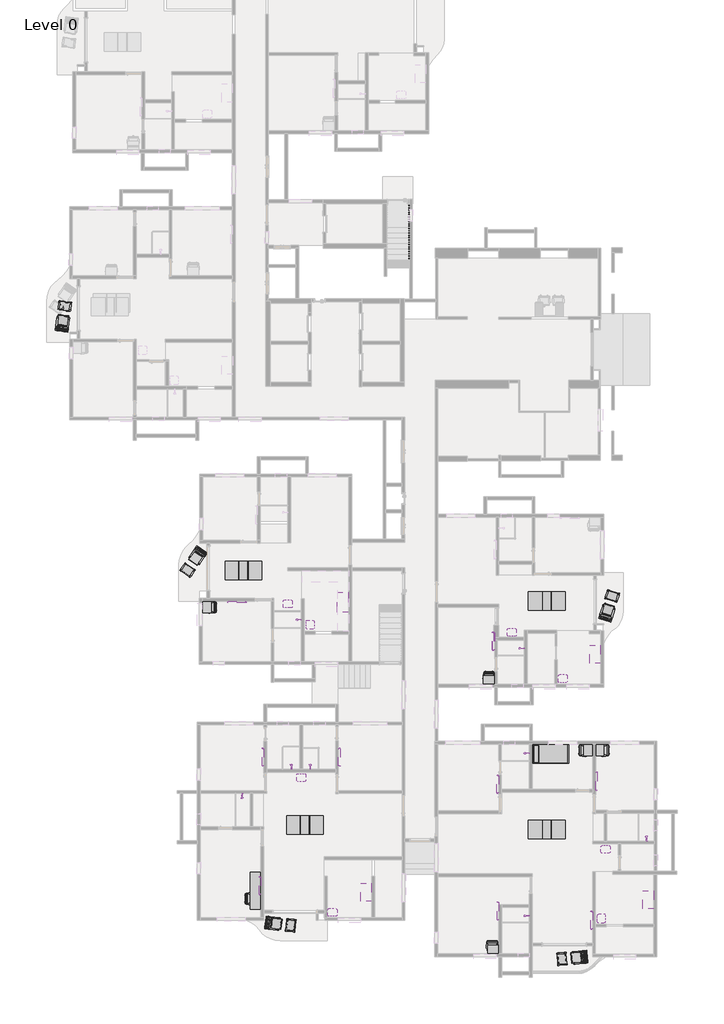
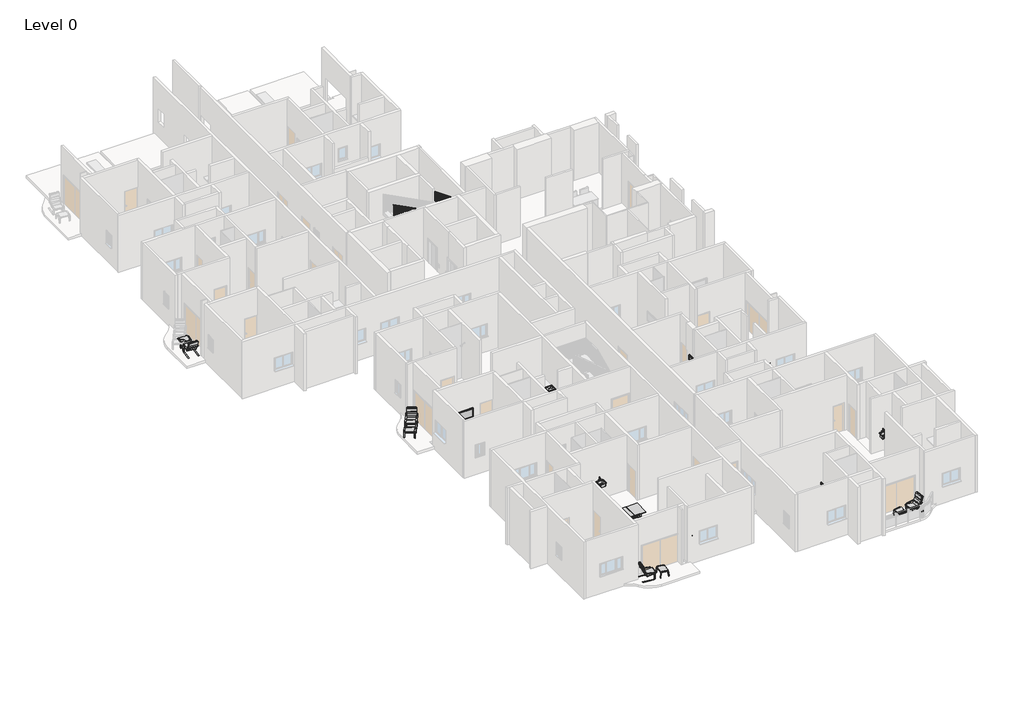
# One storey, part 13 of 14: 32 furniture elements, 16 flow terminals, 4 proxies, 1 railing.
"""IFC4 building model written with IfcOpenShell, lengths in millimetres."""

from ifc_helpers import new_model, si_unit, frame, origin, place, context, project, spatial, polyline, outline, extrude, faceted_brep, transform, mapped, element, save
from components import cook_top_2_0915_x_500mm_892363c5, cook_top_2_1000_x_525mm_c9be7e00, flow_terminal_f629513f, plumbing_fixtures_shower_head_metal_shower_head_9404fff0, furniture_b0964881, furniture_8acf2248, escritorio_de_estudiante_de_600x740mm_600_x_460_x_740mm_3f482482, furniture_bed_2_1040x1981x330mm_twin_f17094d1, furniture_chair_desk_w_armrest_2_635x686x380mm_bb362225, furniture_0b97a49d, furniture_table_dining_w_chairs_rectangular_2000x1000x750mm_b8cbee69

model = new_model("IFC4")

# Units and contexts
model_context = context("Model", 3, world=origin())
ifc_project = project(units=[si_unit("LENGTHUNIT", "METRE", prefix="MILLI")], contexts=[model_context])

# Site, building, storey
site = spatial("IfcSite", under=ifc_project)
building = spatial("IfcBuilding", under=site)
storey = spatial("IfcBuildingStorey", under=building, Name="Level 0", Elevation=0.0)

# Proxies
placement = place(None, origin())
cook_top_2_0915_x_500mm_shape = cook_top_2_0915_x_500mm_892363c5(model_context)
element("IfcBuildingElementProxy", 1, Name="Cook_Top_(2) : 0915 x 500mm", ObjectType="Cook_Top_(2) : 0915 x 500mm", at=placement, inside=storey, context=model_context, shape_type="MappedRepresentation", body=[
    mapped(cook_top_2_0915_x_500mm_shape, transform((-23700.2563508, 13394.0304681, 457.2), x_axis=(0.0, 1.0, 0.0), y_axis=(-1.0, 0.0, 0.0), z_axis=(0.0, 0.0, 1.0))),
])
element("IfcBuildingElementProxy", 2, Name="Cook_Top_(2) : 0915 x 500mm", ObjectType="Cook_Top_(2) : 0915 x 500mm", at=placement, inside=storey, context=model_context, shape_type="MappedRepresentation", body=[
    mapped(cook_top_2_0915_x_500mm_shape, transform((-8354.9935991, 12985.3236639, 457.2), x_axis=(0.0, 1.0, 0.0), y_axis=(-1.0, 0.0, 0.0), z_axis=(0.0, 0.0, 1.0))),
])
element("IfcBuildingElementProxy", 3, Name="Cook_Top_(2) : 0915 x 500mm", ObjectType="Cook_Top_(2) : 0915 x 500mm", at=placement, inside=storey, context=model_context, shape_type="MappedRepresentation", body=[
    mapped(cook_top_2_0915_x_500mm_shape, transform((-11246.4933798, 26344.7122683, 457.2), x_axis=(0.0, 1.0, 0.0), y_axis=(-1.0, 0.0, 0.0), z_axis=(0.0, 0.0, 1.0))),
])
cook_top_2_1000_x_525mm_shape = cook_top_2_1000_x_525mm_c9be7e00(model_context)
element("IfcBuildingElementProxy", 4, Name="Cook_Top_(2) : 1000 x 525mm", ObjectType="Cook_Top_(2) : 1000 x 525mm", at=placement, inside=storey, context=model_context, shape_type="MappedRepresentation", body=[
    mapped(cook_top_2_1000_x_525mm_shape, transform((-24977.1800447, 29166.6991476, 457.2), x_axis=(0.0, 1.0, 0.0), y_axis=(-1.0, 0.0, 0.0), z_axis=(0.0, 0.0, 1.0))),
])

# Flow terminals
flow_terminal_shape = flow_terminal_f629513f(model_context)
element("IfcFlowTerminal", 5, at=placement, inside=storey, context=model_context, shape_type="MappedRepresentation", body=[
    mapped(flow_terminal_shape, transform((-27939.6408041, 29039.3966757, 762.0), x_axis=(-1.0, 0.0, 0.0), y_axis=(0.0, -1.0, 0.0), z_axis=(0.0, 0.0, 1.0))),
])
element("IfcFlowTerminal", 6, at=placement, inside=storey, context=model_context, shape_type="MappedRepresentation", body=[
    mapped(flow_terminal_shape, transform((-26782.1487177, 27927.4094341, 762.0), x_axis=(0.0, 1.0, 0.0), y_axis=(-1.0, 0.0, 0.0), z_axis=(0.0, 0.0, 1.0))),
])
element("IfcFlowTerminal", 7, at=placement, inside=storey, context=model_context, shape_type="MappedRepresentation", body=[
    mapped(flow_terminal_shape, transform((-25513.3671102, 12262.5004802, 762.0), x_axis=(-1.0, 0.0, 0.0), y_axis=(0.0, -1.0, 0.0), z_axis=(0.0, 0.0, 1.0))),
])
element("IfcFlowTerminal", 8, at=placement, inside=storey, context=model_context, shape_type="MappedRepresentation", body=[
    mapped(flow_terminal_shape, transform((-27246.6966639, 19668.6207871, 762.0), x_axis=(1.0, 0.0, 0.0), y_axis=(0.0, 1.0, 0.0), z_axis=(0.0, 0.0, 1.0))),
])
element("IfcFlowTerminal", 9, at=placement, inside=storey, context=model_context, shape_type="MappedRepresentation", body=[
    mapped(flow_terminal_shape, transform((-10697.2845733, 15763.9326754, 762.0), x_axis=(1.0, 0.0, 0.0), y_axis=(0.0, 1.0, 0.0), z_axis=(0.0, 0.0, 1.0))),
])
element("IfcFlowTerminal", 10, at=placement, inside=storey, context=model_context, shape_type="MappedRepresentation", body=[
    mapped(flow_terminal_shape, transform((-10940.2731979, 11953.6344233, 762.0), x_axis=(0.0, 1.0, 0.0), y_axis=(-1.0, 0.0, 0.0), z_axis=(0.0, 0.0, 1.0))),
])
element("IfcFlowTerminal", 11, at=placement, inside=storey, context=model_context, shape_type="MappedRepresentation", body=[
    mapped(flow_terminal_shape, transform((-12991.7531767, 24978.6326694, 762.0), x_axis=(-1.0, 0.0, 0.0), y_axis=(0.0, -1.0, 0.0), z_axis=(0.0, 0.0, 1.0))),
])
element("IfcFlowTerminal", 12, at=placement, inside=storey, context=model_context, shape_type="MappedRepresentation", body=[
    mapped(flow_terminal_shape, transform((-15758.2525392, 27493.2326694, 762.0), x_axis=(-1.0, 0.0, 0.0), y_axis=(0.0, -1.0, 0.0), z_axis=(0.0, 0.0, 1.0))),
])
plumbing_fixtures_shower_head_metal_shower_head_shape = plumbing_fixtures_shower_head_metal_shower_head_9404fff0(model_context)
element("IfcFlowTerminal", 13, ObjectType="Plumbing_Fixtures_Shower_Head : Metal_Shower_Head", at=placement, inside=storey, context=model_context, shape_type="MappedRepresentation", body=[
    mapped(plumbing_fixtures_shower_head_metal_shower_head_shape, transform((-27219.4691188, 28222.4986746, 1369.1616), x_axis=(0.0, 1.0, 0.0), y_axis=(-1.0, 0.0, 0.0), z_axis=(0.0, 0.0, 1.0))),
])
element("IfcFlowTerminal", 14, ObjectType="Plumbing_Fixtures_Shower_Head : Metal_Shower_Head", at=placement, inside=storey, context=model_context, shape_type="MappedRepresentation", body=[
    mapped(plumbing_fixtures_shower_head_metal_shower_head_shape, transform((-27764.4074234, 20080.5411882, 1369.1616), x_axis=(1.0, 0.0, 0.0), y_axis=(0.0, 1.0, 0.0), z_axis=(0.0, 0.0, 1.0))),
])
element("IfcFlowTerminal", 15, ObjectType="Plumbing_Fixtures_Shower_Head : Metal_Shower_Head", at=placement, inside=storey, context=model_context, shape_type="MappedRepresentation", body=[
    mapped(plumbing_fixtures_shower_head_metal_shower_head_shape, transform((-26739.6814081, 20080.5411882, 1219.2), x_axis=(1.0, 0.0, 0.0), y_axis=(0.0, 1.0, 0.0), z_axis=(0.0, 0.0, 1.0))),
])
element("IfcFlowTerminal", 16, ObjectType="Plumbing_Fixtures_Shower_Head : Metal_Shower_Head", at=placement, inside=storey, context=model_context, shape_type="MappedRepresentation", body=[
    mapped(plumbing_fixtures_shower_head_metal_shower_head_shape, transform((-30442.5632392, 18766.3601529, 1369.1616), x_axis=(-1.0, 0.0, 0.0), y_axis=(0.0, -1.0, 0.0), z_axis=(0.0, 0.0, 1.0))),
])
element("IfcFlowTerminal", 17, ObjectType="Plumbing_Fixtures_Shower_Head : Metal_Shower_Head", at=placement, inside=storey, context=model_context, shape_type="MappedRepresentation", body=[
    mapped(plumbing_fixtures_shower_head_metal_shower_head_shape, transform((-14815.4433343, 12112.2999087, 1369.1616), x_axis=(0.0, 1.0, 0.0), y_axis=(-1.0, 0.0, 0.0), z_axis=(0.0, 0.0, 1.0))),
])
element("IfcFlowTerminal", 18, ObjectType="Plumbing_Fixtures_Shower_Head : Metal_Shower_Head", at=placement, inside=storey, context=model_context, shape_type="MappedRepresentation", body=[
    mapped(plumbing_fixtures_shower_head_metal_shower_head_shape, transform((-14822.8537173, 20959.9122683, 1219.2), x_axis=(0.0, 1.0, 0.0), y_axis=(-1.0, 0.0, 0.0), z_axis=(0.0, 0.0, 1.0))),
])
element("IfcFlowTerminal", 19, ObjectType="Plumbing_Fixtures_Shower_Head : Metal_Shower_Head", at=placement, inside=storey, context=model_context, shape_type="MappedRepresentation", body=[
    mapped(plumbing_fixtures_shower_head_metal_shower_head_shape, transform((-8446.3933343, 16175.8530766, 1219.2), x_axis=(1.0, 0.0, 0.0), y_axis=(0.0, 1.0, 0.0), z_axis=(0.0, 0.0, 1.0))),
])
element("IfcFlowTerminal", 20, ObjectType="Plumbing_Fixtures_Shower_Head : Metal_Shower_Head", at=placement, inside=storey, context=model_context, shape_type="MappedRepresentation", body=[
    mapped(plumbing_fixtures_shower_head_metal_shower_head_shape, transform((-15090.4456172, 26659.159605, 1369.1616), x_axis=(0.0, 1.0, 0.0), y_axis=(-1.0, 0.0, 0.0), z_axis=(0.0, 0.0, 1.0))),
])

# Furniture
furniture_shape = furniture_b0964881(model_context)
element("IfcFurniture", 21, at=placement, inside=storey, context=model_context, shape_type="MappedRepresentation", body=[
    mapped(furniture_shape, transform((-32860.2351319, 31699.8029421, 149.9616), x_axis=(-0.8191520442889915, 0.5735764363510468, 0.0), y_axis=(-0.5735764363510468, -0.8191520442889915, 0.0), z_axis=(0.0, 0.0, 1.0))),
])
element("IfcFurniture", 22, at=placement, inside=storey, context=model_context, shape_type="MappedRepresentation", body=[
    mapped(furniture_shape, transform((-28756.835076, 11705.9130648, 149.9616), x_axis=(-0.11901565974677361, -0.9928923772167054, 0.0), y_axis=(0.9928923772167054, -0.11901565974677361, 0.0), z_axis=(0.0, 0.0, 1.0))),
])
element("IfcFurniture", 23, at=placement, inside=storey, context=model_context, shape_type="MappedRepresentation", body=[
    mapped(furniture_shape, transform((-12089.4158343, 9854.1185188, 149.9616), x_axis=(-0.09003022403644445, 0.995939033656151, 0.0), y_axis=(-0.995939033656151, -0.09003022403644445, 0.0), z_axis=(0.0, 0.0, 1.0))),
])
element("IfcFurniture", 24, at=placement, inside=storey, context=model_context, shape_type="MappedRepresentation", body=[
    mapped(furniture_shape, transform((-10596.425027, 28588.0695695, 149.9616), x_axis=(0.9563047559630339, -0.29237170472274204, 0.0), y_axis=(0.29237170472274204, 0.9563047559630339, 0.0), z_axis=(0.0, 0.0, 1.0))),
])
element("IfcFurniture", 25, at=placement, inside=storey, context=model_context, shape_type="MappedRepresentation", body=[
    mapped(furniture_shape, transform((-40209.0307664, 44321.306806, 149.9616), x_axis=(0.9925461516413222, -0.1218693434051461, 0.0), y_axis=(0.1218693434051461, 0.9925461516413222, 0.0), z_axis=(0.0, 0.0, 1.0))),
])
furniture_2_shape = furniture_8acf2248(model_context)
element("IfcFurniture", 26, at=placement, inside=storey, context=model_context, shape_type="MappedRepresentation", body=[
    mapped(furniture_2_shape, transform((-29421.6063508, 14488.3294818, 149.9616), x_axis=(0.0, -1.0, 0.0), y_axis=(1.0, 0.0, 0.0), z_axis=(0.0, 0.0, 1.0))),
])
escritorio_de_estudiante_de_600x740mm_600_x_460_x_740mm_shape = escritorio_de_estudiante_de_600x740mm_600_x_460_x_740mm_3f482482(model_context)
element("IfcFurniture", 27, ObjectType="Escritorio_de_estudiante_de_600x740mm : 600 x 460 x 740mm", at=placement, inside=storey, context=model_context, shape_type="MappedRepresentation", body=[
    mapped(escritorio_de_estudiante_de_600x740mm_600_x_460_x_740mm_shape, transform((-32355.8800447, 28900.5770746, 149.9616), x_axis=(0.0, 1.0, 0.0), y_axis=(-1.0, 0.0, 0.0), z_axis=(0.0, 0.0, 1.0))),
])
element("IfcFurniture", 28, ObjectType="Escritorio_de_estudiante_de_600x740mm : 600 x 460 x 740mm", at=placement, inside=storey, context=model_context, shape_type="MappedRepresentation", body=[
    mapped(escritorio_de_estudiante_de_600x740mm_600_x_460_x_740mm_shape, transform((-16781.6276027, 10272.6590683, 149.9616), x_axis=(1.0, 0.0, 0.0), y_axis=(0.0, 1.0, 0.0), z_axis=(0.0, 0.0, 1.0))),
])
element("IfcFurniture", 29, ObjectType="Escritorio_de_estudiante_de_600x740mm : 600 x 460 x 740mm", at=placement, inside=storey, context=model_context, shape_type="MappedRepresentation", body=[
    mapped(escritorio_de_estudiante_de_600x740mm_600_x_460_x_740mm_shape, transform((-11622.4537173, 21112.3122683, 149.9616), x_axis=(0.0, 1.0, 0.0), y_axis=(-1.0, 0.0, 0.0), z_axis=(0.0, 0.0, 1.0))),
])
element("IfcFurniture", 30, ObjectType="Escritorio_de_estudiante_de_600x740mm : 600 x 460 x 740mm", at=placement, inside=storey, context=model_context, shape_type="MappedRepresentation", body=[
    mapped(escritorio_de_estudiante_de_600x740mm_600_x_460_x_740mm_shape, transform((-10994.5465173, 21112.3122683, 149.9616), x_axis=(0.0, 1.0, 0.0), y_axis=(-1.0, 0.0, 0.0), z_axis=(0.0, 0.0, 1.0))),
])
element("IfcFurniture", 31, ObjectType="Escritorio_de_estudiante_de_600x740mm : 600 x 460 x 740mm", at=placement, inside=storey, context=model_context, shape_type="MappedRepresentation", body=[
    mapped(escritorio_de_estudiante_de_600x740mm_600_x_460_x_740mm_shape, transform((-17020.8456172, 24931.959605, 149.9616), x_axis=(1.0, 0.0, 0.0), y_axis=(0.0, 1.0, 0.0), z_axis=(0.0, 0.0, 1.0))),
])
furniture_bed_2_1040x1981x330mm_twin_shape = furniture_bed_2_1040x1981x330mm_twin_f17094d1(model_context)
element("IfcFurniture", 32, ObjectType="Furniture_Bed_2 : 1040x1981x330mm-Twin", at=placement, inside=storey, context=model_context, shape_type="MappedRepresentation", body=[
    mapped(furniture_bed_2_1040x1981x330mm_twin_shape, transform((-14670.4537173, 20940.8622683, 149.9616), x_axis=(0.0, 1.0, 0.0), y_axis=(-1.0, 0.0, 0.0), z_axis=(0.0, 0.0, 1.0))),
])
furniture_chair_desk_w_armrest_2_635x686x380mm_shape = furniture_chair_desk_w_armrest_2_635x686x380mm_bb362225(model_context)
element("IfcFurniture", 33, ObjectType="Furniture_Chair_Desk_w-Armrest_2 : 635x686x380mm", at=placement, inside=storey, context=model_context, shape_type="MappedRepresentation", body=[
    mapped(furniture_chair_desk_w_armrest_2_635x686x380mm_shape, transform((-32106.9341431, 28759.586255, 149.9616), x_axis=(0.0, 1.0, 0.0), y_axis=(-1.0, 0.0, 0.0), z_axis=(0.0, 0.0, 1.0))),
])
element("IfcFurniture", 34, ObjectType="Furniture_Chair_Desk_w-Armrest_2 : 635x686x380mm", at=placement, inside=storey, context=model_context, shape_type="MappedRepresentation", body=[
    mapped(furniture_chair_desk_w_armrest_2_635x686x380mm_shape, transform((-30021.5772524, 13185.3708988, 149.9616), x_axis=(0.0, -1.0, 0.0), y_axis=(1.0, 0.0, 0.0), z_axis=(0.0, 0.0, 1.0))),
])
element("IfcFurniture", 35, ObjectType="Furniture_Chair_Desk_w-Armrest_2 : 635x686x380mm", at=placement, inside=storey, context=model_context, shape_type="MappedRepresentation", body=[
    mapped(furniture_chair_desk_w_armrest_2_635x686x380mm_shape, transform((-16700.2041146, 10494.80497, 149.9616), x_axis=(-1.0, 0.0, 0.0), y_axis=(0.0, -1.0, 0.0), z_axis=(0.0, 0.0, 1.0))),
])
element("IfcFurniture", 36, ObjectType="Furniture_Chair_Desk_w-Armrest_2 : 635x686x380mm", at=placement, inside=storey, context=model_context, shape_type="MappedRepresentation", body=[
    mapped(furniture_chair_desk_w_armrest_2_635x686x380mm_shape, transform((-11871.399619, 21253.303088, 149.9616), x_axis=(0.0, -1.0, 0.0), y_axis=(1.0, 0.0, 0.0), z_axis=(0.0, 0.0, 1.0))),
])
element("IfcFurniture", 37, ObjectType="Furniture_Chair_Desk_w-Armrest_2 : 635x686x380mm", at=placement, inside=storey, context=model_context, shape_type="MappedRepresentation", body=[
    mapped(furniture_chair_desk_w_armrest_2_635x686x380mm_shape, transform((-10738.8494311, 20971.3214487, 149.9616), x_axis=(0.0, 1.0, 0.0), y_axis=(-1.0, 0.0, 0.0), z_axis=(0.0, 0.0, 1.0))),
])
element("IfcFurniture", 38, ObjectType="Furniture_Chair_Desk_w-Armrest_2 : 635x686x380mm", at=placement, inside=storey, context=model_context, shape_type="MappedRepresentation", body=[
    mapped(furniture_chair_desk_w_armrest_2_635x686x380mm_shape, transform((-16879.8547976, 25144.45817, 149.9616), x_axis=(-1.0, 0.0, 0.0), y_axis=(0.0, -1.0, 0.0), z_axis=(0.0, 0.0, 1.0))),
])
furniture_3_shape = furniture_0b97a49d(model_context)
element("IfcFurniture", 39, ObjectType="Furniture_TV_Plasma : 42\"", at=placement, inside=storey, context=model_context, shape_type="MappedRepresentation", body=[
    mapped(furniture_3_shape, transform((-30796.9550447, 29230.7770746, 1369.1616), x_axis=(1.0, 0.0, 0.0), y_axis=(0.0, 1.0, 0.0), z_axis=(0.0, 0.0, 1.0))),
])
element("IfcFurniture", 40, ObjectType="Furniture_TV_Plasma : 42\"", at=placement, inside=storey, context=model_context, shape_type="MappedRepresentation", body=[
    mapped(furniture_3_shape, transform((-29421.6063508, 13796.1794818, 1369.1616), x_axis=(0.0, -1.0, 0.0), y_axis=(1.0, 0.0, 0.0), z_axis=(0.0, 0.0, 1.0))),
])
element("IfcFurniture", 41, ObjectType="Furniture_TV_Plasma : 42\"", at=placement, inside=storey, context=model_context, shape_type="MappedRepresentation", body=[
    mapped(furniture_3_shape, transform((-29259.4280604, 20804.4411882, 1369.1616), x_axis=(0.0, -1.0, 0.0), y_axis=(1.0, 0.0, 0.0), z_axis=(0.0, 0.0, 1.0))),
])
element("IfcFurniture", 42, ObjectType="Furniture_TV_Plasma : 42\"", at=placement, inside=storey, context=model_context, shape_type="MappedRepresentation", body=[
    mapped(furniture_3_shape, transform((-25206.9553928, 20690.1411882, 1369.1616), x_axis=(0.0, 1.0, 0.0), y_axis=(-1.0, 0.0, 0.0), z_axis=(0.0, 0.0, 1.0))),
])
element("IfcFurniture", 43, ObjectType="Furniture_TV_Plasma : 42\"", at=placement, inside=storey, context=model_context, shape_type="MappedRepresentation", body=[
    mapped(furniture_3_shape, transform((-16476.8276027, 12429.7999087, 1219.2), x_axis=(0.0, -1.0, 0.0), y_axis=(1.0, 0.0, 0.0), z_axis=(0.0, 0.0, 1.0))),
])
element("IfcFurniture", 44, ObjectType="Furniture_TV_Plasma : 42\"", at=placement, inside=storey, context=model_context, shape_type="MappedRepresentation", body=[
    mapped(furniture_3_shape, transform((-11223.1465173, 19372.4122683, 1369.1616), x_axis=(0.0, 1.0, 0.0), y_axis=(-1.0, 0.0, 0.0), z_axis=(0.0, 0.0, 1.0))),
])
element("IfcFurniture", 45, ObjectType="Furniture_TV_Plasma : 42\"", at=placement, inside=storey, context=model_context, shape_type="MappedRepresentation", body=[
    mapped(furniture_3_shape, transform((-16492.0741157, 19327.9114683, 1369.1616), x_axis=(0.0, -1.0, 0.0), y_axis=(1.0, 0.0, 0.0), z_axis=(0.0, 0.0, 1.0))),
])
element("IfcFurniture", 46, ObjectType="Furniture_TV_Plasma : 42\"", at=placement, inside=storey, context=model_context, shape_type="MappedRepresentation", body=[
    mapped(furniture_3_shape, transform((-16745.0362231, 27094.0122683, 1369.1616), x_axis=(0.0, -1.0, 0.0), y_axis=(1.0, 0.0, 0.0), z_axis=(0.0, 0.0, 1.0))),
])
element("IfcFurniture", 47, ObjectType="Furniture_TV_Plasma : 42\"", at=placement, inside=storey, context=model_context, shape_type="MappedRepresentation", body=[
    mapped(furniture_3_shape, transform((-11377.5935991, 11936.3590683, 1369.1616), x_axis=(0.0, -1.0, 0.0), y_axis=(1.0, 0.0, 0.0), z_axis=(0.0, 0.0, 1.0))),
])
element("IfcFurniture", 48, ObjectType="Furniture_TV_Plasma : 42\"", at=placement, inside=storey, context=model_context, shape_type="MappedRepresentation", body=[
    mapped(furniture_3_shape, transform((-16716.0456172, 27094.0122683, 1369.1616), x_axis=(0.0, -1.0, 0.0), y_axis=(1.0, 0.0, 0.0), z_axis=(0.0, 0.0, 1.0))),
])
furniture_table_dining_w_chairs_rectangular_2000x1000x750mm_shape = furniture_table_dining_w_chairs_rectangular_2000x1000x750mm_b8cbee69(model_context)
element("IfcFurniture", 49, ObjectType="Furniture_Table_Dining_w-Chairs_Rectangular : 2000x1000x750mm_w-6_Seats", at=placement, inside=storey, context=model_context, shape_type="MappedRepresentation", body=[
    mapped(furniture_table_dining_w_chairs_rectangular_2000x1000x750mm_shape, transform((-30491.0276487, 30839.6748526, 149.9616), x_axis=(1.0, 0.0, 0.0), y_axis=(0.0, 1.0, 0.0), z_axis=(0.0, 0.0, 1.0))),
])
element("IfcFurniture", 50, ObjectType="Furniture_Table_Dining_w-Chairs_Rectangular : 2000x1000x750mm_w-6_Seats", at=placement, inside=storey, context=model_context, shape_type="MappedRepresentation", body=[
    mapped(furniture_table_dining_w_chairs_rectangular_2000x1000x750mm_shape, transform((-27145.8350726, 17016.5560391, 149.9616), x_axis=(1.0, 0.0, 0.0), y_axis=(0.0, 1.0, 0.0), z_axis=(0.0, 0.0, 1.0))),
])
element("IfcFurniture", 51, ObjectType="Furniture_Table_Dining_w-Chairs_Rectangular : 2000x1000x750mm_w-6_Seats", at=placement, inside=storey, context=model_context, shape_type="MappedRepresentation", body=[
    mapped(furniture_table_dining_w_chairs_rectangular_2000x1000x750mm_shape, transform((-13989.2719391, 16757.15655, 149.9616), x_axis=(1.0, 0.0, 0.0), y_axis=(0.0, 1.0, 0.0), z_axis=(0.0, 0.0, 1.0))),
])
element("IfcFurniture", 52, ObjectType="Furniture_Table_Dining_w-Chairs_Rectangular : 2000x1000x750mm_w-6_Seats", at=placement, inside=storey, context=model_context, shape_type="MappedRepresentation", body=[
    mapped(furniture_table_dining_w_chairs_rectangular_2000x1000x750mm_shape, transform((-13989.2719391, 29186.4224454, 149.9616), x_axis=(1.0, 0.0, 0.0), y_axis=(0.0, 1.0, 0.0), z_axis=(0.0, 0.0, 1.0))),
])

# Railing
element("IfcRailing", 53, ObjectType="1100mm", at=placement, inside=storey, context=model_context, shape_type="SolidModel", body=[
    faceted_brep([(-21345.6288686, 51059.2706597, 1266.6666667), (-21345.6288686, 51059.2706597, 1212.8024595), (-21395.6288686, 51059.2706597, 1212.8024595), (-21395.6288686, 51059.2706597, 1266.6666667), (-21345.6288686, 46940.0134704, 2917.153478), (-21345.6288686, 46930.3692473, 2867.153478), (-21395.6288686, 46930.3692473, 2867.153478), (-21395.6288686, 46940.0134704, 2917.153478), (-21345.6288686, 45662.0690597, 2867.153478), (-21345.6288686, 45662.0690597, 2917.153478), (-22349.9075898, 45662.0690597, 2917.153478), (-22361.9769951, 45662.0690597, 2867.153478), (-21395.6288686, 45712.0690597, 2867.153478), (-22361.9769951, 45712.0690597, 2867.153478), (-21395.6288686, 45712.0690597, 2917.153478), (-22349.9075898, 45712.0690597, 2917.153478), (-25957.6772109, 45662.0690597, 4766.6666667), (-25957.6772109, 45712.0690597, 4766.6666667), (-25957.6772109, 45712.0690597, 4710.4793192), (-25957.6772109, 45662.0690597, 4710.4793192)], [[[0, 1, 2, 3]], [[1, 0, 4, 5]], [[2, 1, 5, 6]], [[3, 2, 6, 7]], [[0, 3, 7, 4]], [[8, 9, 10, 11]], [[12, 8, 11, 13]], [[14, 12, 13, 15]], [[9, 14, 15, 10]], [[5, 4, 9, 8]], [[6, 5, 8, 12]], [[7, 6, 12, 14]], [[4, 7, 14, 9]], [[16, 17, 18, 19]], [[11, 10, 16, 19]], [[13, 11, 19, 18]], [[15, 13, 18, 17]], [[10, 15, 17, 16]]]),
    extrude(outline(polyline([(4691.4865882, -25920.6288686), (4704.3027696, -25945.6288686), (3500.0, -25945.6288686), (3500.0, -25920.6288686), (4691.4865882, -25920.6288686)])), frame((0.0, 45674.5690597, 0.0), z_axis=(0.0, 1.0, 0.0), x_axis=(0.0, 0.0, 1.0)), (0.0, 0.0, 1.0), 25.0),
    extrude(outline(polyline([(4627.4056815, -25795.6288686), (4640.2218629, -25820.6288686), (3500.0, -25820.6288686), (3500.0, -25795.6288686), (4627.4056815, -25795.6288686)])), frame((0.0, 45674.5690597, 0.0), z_axis=(0.0, 1.0, 0.0), x_axis=(0.0, 0.0, 1.0)), (0.0, 0.0, 1.0), 25.0),
    extrude(outline(polyline([(4563.3247748, -25670.6288686), (4576.1409561, -25695.6288686), (3500.0, -25695.6288686), (3500.0, -25670.6288686), (4563.3247748, -25670.6288686)])), frame((0.0, 45674.5690597, 0.0), z_axis=(0.0, 1.0, 0.0), x_axis=(0.0, 0.0, 1.0)), (0.0, 0.0, 1.0), 25.0),
    extrude(outline(polyline([(4499.2438681, -25545.6288686), (4512.0600494, -25570.6288686), (3333.3333333, -25570.6288686), (3333.3333333, -25545.6288686), (4499.2438681, -25545.6288686)])), frame((0.0, 45674.5690597, 0.0), z_axis=(0.0, 1.0, 0.0), x_axis=(0.0, 0.0, 1.0)), (0.0, 0.0, 1.0), 25.0),
    extrude(outline(polyline([(4435.1629613, -25420.6288686), (4447.9791427, -25445.6288686), (3333.3333333, -25445.6288686), (3333.3333333, -25420.6288686), (4435.1629613, -25420.6288686)])), frame((0.0, 45674.5690597, 0.0), z_axis=(0.0, 1.0, 0.0), x_axis=(0.0, 0.0, 1.0)), (0.0, 0.0, 1.0), 25.0),
    extrude(outline(polyline([(4371.0820546, -25295.6288686), (4383.8982359, -25320.6288686), (3166.6666667, -25320.6288686), (3166.6666667, -25295.6288686), (4371.0820546, -25295.6288686)])), frame((0.0, 45674.5690597, 0.0), z_axis=(0.0, 1.0, 0.0), x_axis=(0.0, 0.0, 1.0)), (0.0, 0.0, 1.0), 25.0),
    extrude(outline(polyline([(4307.0011479, -25170.6288686), (4319.8173292, -25195.6288686), (3166.6666667, -25195.6288686), (3166.6666667, -25170.6288686), (4307.0011479, -25170.6288686)])), frame((0.0, 45674.5690597, 0.0), z_axis=(0.0, 1.0, 0.0), x_axis=(0.0, 0.0, 1.0)), (0.0, 0.0, 1.0), 25.0),
    extrude(outline(polyline([(4242.9202411, -25045.6288686), (4255.7364225, -25070.6288686), (3000.0, -25070.6288686), (3000.0, -25045.6288686), (4242.9202411, -25045.6288686)])), frame((0.0, 45674.5690597, 0.0), z_axis=(0.0, 1.0, 0.0), x_axis=(0.0, 0.0, 1.0)), (0.0, 0.0, 1.0), 25.0),
    extrude(outline(polyline([(4178.8393344, -24920.6288686), (4191.6555158, -24945.6288686), (3000.0, -24945.6288686), (3000.0, -24920.6288686), (4178.8393344, -24920.6288686)])), frame((0.0, 45674.5690597, 0.0), z_axis=(0.0, 1.0, 0.0), x_axis=(0.0, 0.0, 1.0)), (0.0, 0.0, 1.0), 25.0),
    extrude(outline(polyline([(4114.7584277, -24795.6288686), (4127.574609, -24820.6288686), (3000.0, -24820.6288686), (3000.0, -24795.6288686), (4114.7584277, -24795.6288686)])), frame((0.0, 45674.5690597, 0.0), z_axis=(0.0, 1.0, 0.0), x_axis=(0.0, 0.0, 1.0)), (0.0, 0.0, 1.0), 25.0),
    extrude(outline(polyline([(4050.677521, -24670.6288686), (4063.4937023, -24695.6288686), (2833.3333333, -24695.6288686), (2833.3333333, -24670.6288686), (4050.677521, -24670.6288686)])), frame((0.0, 45674.5690597, 0.0), z_axis=(0.0, 1.0, 0.0), x_axis=(0.0, 0.0, 1.0)), (0.0, 0.0, 1.0), 25.0),
    extrude(outline(polyline([(3986.5966142, -24545.6288686), (3999.4127956, -24570.6288686), (2833.3333333, -24570.6288686), (2833.3333333, -24545.6288686), (3986.5966142, -24545.6288686)])), frame((0.0, 45674.5690597, 0.0), z_axis=(0.0, 1.0, 0.0), x_axis=(0.0, 0.0, 1.0)), (0.0, 0.0, 1.0), 25.0),
    extrude(outline(polyline([(3922.5157075, -24420.6288686), (3935.3318888, -24445.6288686), (2666.6666667, -24445.6288686), (2666.6666667, -24420.6288686), (3922.5157075, -24420.6288686)])), frame((0.0, 45674.5690597, 0.0), z_axis=(0.0, 1.0, 0.0), x_axis=(0.0, 0.0, 1.0)), (0.0, 0.0, 1.0), 25.0),
    extrude(outline(polyline([(3858.4348008, -24295.6288686), (3871.2509821, -24320.6288686), (2666.6666667, -24320.6288686), (2666.6666667, -24295.6288686), (3858.4348008, -24295.6288686)])), frame((0.0, 45674.5690597, 0.0), z_axis=(0.0, 1.0, 0.0), x_axis=(0.0, 0.0, 1.0)), (0.0, 0.0, 1.0), 25.0),
    extrude(outline(polyline([(3794.353894, -24170.6288686), (3807.1700754, -24195.6288686), (2666.6666667, -24195.6288686), (2666.6666667, -24170.6288686), (3794.353894, -24170.6288686)])), frame((0.0, 45674.5690597, 0.0), z_axis=(0.0, 1.0, 0.0), x_axis=(0.0, 0.0, 1.0)), (0.0, 0.0, 1.0), 25.0),
    extrude(outline(polyline([(3730.2729873, -24045.6288686), (3743.0891687, -24070.6288686), (2500.0, -24070.6288686), (2500.0, -24045.6288686), (3730.2729873, -24045.6288686)])), frame((0.0, 45674.5690597, 0.0), z_axis=(0.0, 1.0, 0.0), x_axis=(0.0, 0.0, 1.0)), (0.0, 0.0, 1.0), 25.0),
    extrude(outline(polyline([(3666.1920806, -23920.6288686), (3679.0082619, -23945.6288686), (2500.0, -23945.6288686), (2500.0, -23920.6288686), (3666.1920806, -23920.6288686)])), frame((0.0, 45674.5690597, 0.0), z_axis=(0.0, 1.0, 0.0), x_axis=(0.0, 0.0, 1.0)), (0.0, 0.0, 1.0), 25.0),
    extrude(outline(polyline([(3602.1111739, -23795.6288686), (3614.9273552, -23820.6288686), (2333.3333333, -23820.6288686), (2333.3333333, -23795.6288686), (3602.1111739, -23795.6288686)])), frame((0.0, 45674.5690597, 0.0), z_axis=(0.0, 1.0, 0.0), x_axis=(0.0, 0.0, 1.0)), (0.0, 0.0, 1.0), 25.0),
    extrude(outline(polyline([(3538.0302671, -23670.6288686), (3550.8464485, -23695.6288686), (2333.3333333, -23695.6288686), (2333.3333333, -23670.6288686), (3538.0302671, -23670.6288686)])), frame((0.0, 45674.5690597, 0.0), z_axis=(0.0, 1.0, 0.0), x_axis=(0.0, 0.0, 1.0)), (0.0, 0.0, 1.0), 25.0),
    extrude(outline(polyline([(3473.9493604, -23545.6288686), (3486.7655418, -23570.6288686), (2166.6666667, -23570.6288686), (2166.6666667, -23545.6288686), (3473.9493604, -23545.6288686)])), frame((0.0, 45674.5690597, 0.0), z_axis=(0.0, 1.0, 0.0), x_axis=(0.0, 0.0, 1.0)), (0.0, 0.0, 1.0), 25.0),
    extrude(outline(polyline([(3409.8684537, -23420.6288686), (3422.684635, -23445.6288686), (2166.6666667, -23445.6288686), (2166.6666667, -23420.6288686), (3409.8684537, -23420.6288686)])), frame((0.0, 45674.5690597, 0.0), z_axis=(0.0, 1.0, 0.0), x_axis=(0.0, 0.0, 1.0)), (0.0, 0.0, 1.0), 25.0),
    extrude(outline(polyline([(3345.787547, -23295.6288686), (3358.6037283, -23320.6288686), (2166.6666667, -23320.6288686), (2166.6666667, -23295.6288686), (3345.787547, -23295.6288686)])), frame((0.0, 45674.5690597, 0.0), z_axis=(0.0, 1.0, 0.0), x_axis=(0.0, 0.0, 1.0)), (0.0, 0.0, 1.0), 25.0),
    extrude(outline(polyline([(3281.7066402, -23170.6288686), (3294.5228216, -23195.6288686), (2166.6666667, -23195.6288686), (2166.6666667, -23170.6288686), (3281.7066402, -23170.6288686)])), frame((0.0, 45674.5690597, 0.0), z_axis=(0.0, 1.0, 0.0), x_axis=(0.0, 0.0, 1.0)), (0.0, 0.0, 1.0), 25.0),
    extrude(outline(polyline([(3217.6257335, -23045.6288686), (3230.4419148, -23070.6288686), (2166.6666667, -23070.6288686), (2166.6666667, -23045.6288686), (3217.6257335, -23045.6288686)])), frame((0.0, 45674.5690597, 0.0), z_axis=(0.0, 1.0, 0.0), x_axis=(0.0, 0.0, 1.0)), (0.0, 0.0, 1.0), 25.0),
    extrude(outline(polyline([(3153.5448268, -22920.6288686), (3166.3610081, -22945.6288686), (2000.0, -22945.6288686), (2000.0, -22920.6288686), (3153.5448268, -22920.6288686)])), frame((0.0, 45674.5690597, 0.0), z_axis=(0.0, 1.0, 0.0), x_axis=(0.0, 0.0, 1.0)), (0.0, 0.0, 1.0), 25.0),
    extrude(outline(polyline([(3089.46392, -22795.6288686), (3102.2801014, -22820.6288686), (2000.0, -22820.6288686), (2000.0, -22795.6288686), (3089.46392, -22795.6288686)])), frame((0.0, 45674.5690597, 0.0), z_axis=(0.0, 1.0, 0.0), x_axis=(0.0, 0.0, 1.0)), (0.0, 0.0, 1.0), 25.0),
    extrude(outline(polyline([(3025.3830133, -22670.6288686), (3038.1991947, -22695.6288686), (1833.3333333, -22695.6288686), (1833.3333333, -22670.6288686), (3025.3830133, -22670.6288686)])), frame((0.0, 45674.5690597, 0.0), z_axis=(0.0, 1.0, 0.0), x_axis=(0.0, 0.0, 1.0)), (0.0, 0.0, 1.0), 25.0),
    extrude(outline(polyline([(2961.3021066, -22545.6288686), (2974.1182879, -22570.6288686), (1833.3333333, -22570.6288686), (1833.3333333, -22545.6288686), (2961.3021066, -22545.6288686)])), frame((0.0, 45674.5690597, 0.0), z_axis=(0.0, 1.0, 0.0), x_axis=(0.0, 0.0, 1.0)), (0.0, 0.0, 1.0), 25.0),
    extrude(outline(polyline([(2897.2211999, -22420.6288686), (2910.0373812, -22445.6288686), (1833.3333333, -22445.6288686), (1833.3333333, -22420.6288686), (2897.2211999, -22420.6288686)])), frame((0.0, 45674.5690597, 0.0), z_axis=(0.0, 1.0, 0.0), x_axis=(0.0, 0.0, 1.0)), (0.0, 0.0, 1.0), 25.0),
    extrude(outline(polyline([(-22295.6288686, 45674.5690597), (-22320.6288686, 45674.5690597), (-22320.6288686, 45699.5690597), (-22295.6288686, 45699.5690597), (-22295.6288686, 45674.5690597)])), frame((0.0, 0.0, 1833.3333333), z_axis=(0.0, 0.0, 1.0), x_axis=(1.0, 0.0, 0.0)), (0.0, 0.0, 1.0), 1033.8201447),
    extrude(outline(polyline([(-22170.6288686, 45674.5690597), (-22195.6288686, 45674.5690597), (-22195.6288686, 45699.5690597), (-22170.6288686, 45699.5690597), (-22170.6288686, 45674.5690597)])), frame((0.0, 0.0, 1833.3333333), z_axis=(0.0, 0.0, 1.0), x_axis=(1.0, 0.0, 0.0)), (0.0, 0.0, 1.0), 1033.8201447),
    extrude(outline(polyline([(-22045.6288686, 45674.5690597), (-22070.6288686, 45674.5690597), (-22070.6288686, 45699.5690597), (-22045.6288686, 45699.5690597), (-22045.6288686, 45674.5690597)])), frame((0.0, 0.0, 1833.3333333), z_axis=(0.0, 0.0, 1.0), x_axis=(1.0, 0.0, 0.0)), (0.0, 0.0, 1.0), 1033.8201447),
    extrude(outline(polyline([(-21920.6288686, 45674.5690597), (-21945.6288686, 45674.5690597), (-21945.6288686, 45699.5690597), (-21920.6288686, 45699.5690597), (-21920.6288686, 45674.5690597)])), frame((0.0, 0.0, 1833.3333333), z_axis=(0.0, 0.0, 1.0), x_axis=(1.0, 0.0, 0.0)), (0.0, 0.0, 1.0), 1033.8201447),
    extrude(outline(polyline([(-21795.6288686, 45674.5690597), (-21820.6288686, 45674.5690597), (-21820.6288686, 45699.5690597), (-21795.6288686, 45699.5690597), (-21795.6288686, 45674.5690597)])), frame((0.0, 0.0, 1833.3333333), z_axis=(0.0, 0.0, 1.0), x_axis=(1.0, 0.0, 0.0)), (0.0, 0.0, 1.0), 1033.8201447),
    extrude(outline(polyline([(-21670.6288686, 45674.5690597), (-21695.6288686, 45674.5690597), (-21695.6288686, 45699.5690597), (-21670.6288686, 45699.5690597), (-21670.6288686, 45674.5690597)])), frame((0.0, 0.0, 1833.3333333), z_axis=(0.0, 0.0, 1.0), x_axis=(1.0, 0.0, 0.0)), (0.0, 0.0, 1.0), 1033.8201447),
    extrude(outline(polyline([(-21545.6288686, 45674.5690597), (-21570.6288686, 45674.5690597), (-21570.6288686, 45699.5690597), (-21545.6288686, 45699.5690597), (-21545.6288686, 45674.5690597)])), frame((0.0, 0.0, 1833.3333333), z_axis=(0.0, 0.0, 1.0), x_axis=(1.0, 0.0, 0.0)), (0.0, 0.0, 1.0), 1033.8201447),
    extrude(outline(polyline([(-21420.6288686, 45674.5690597), (-21445.6288686, 45674.5690597), (-21445.6288686, 45699.5690597), (-21420.6288686, 45699.5690597), (-21420.6288686, 45674.5690597)])), frame((0.0, 0.0, 1833.3333333), z_axis=(0.0, 0.0, 1.0), x_axis=(1.0, 0.0, 0.0)), (0.0, 0.0, 1.0), 1033.8201447),
    extrude(outline(polyline([(-21358.1288686, 45759.2706597), (-21358.1288686, 45734.2706597), (-21383.1288686, 45734.2706597), (-21383.1288686, 45759.2706597), (-21358.1288686, 45759.2706597)])), frame((0.0, 0.0, 1833.3333333), z_axis=(0.0, 0.0, 1.0), x_axis=(1.0, 0.0, 0.0)), (0.0, 0.0, 1.0), 1033.8201447),
    extrude(outline(polyline([(-21358.1288686, 45884.2706597), (-21358.1288686, 45859.2706597), (-21383.1288686, 45859.2706597), (-21383.1288686, 45884.2706597), (-21358.1288686, 45884.2706597)])), frame((0.0, 0.0, 1833.3333333), z_axis=(0.0, 0.0, 1.0), x_axis=(1.0, 0.0, 0.0)), (0.0, 0.0, 1.0), 1033.8201447),
    extrude(outline(polyline([(-21358.1288686, 46009.2706597), (-21358.1288686, 45984.2706597), (-21383.1288686, 45984.2706597), (-21383.1288686, 46009.2706597), (-21358.1288686, 46009.2706597)])), frame((0.0, 0.0, 1833.3333333), z_axis=(0.0, 0.0, 1.0), x_axis=(1.0, 0.0, 0.0)), (0.0, 0.0, 1.0), 1033.8201447),
    extrude(outline(polyline([(-21358.1288686, 46134.2706597), (-21358.1288686, 46109.2706597), (-21383.1288686, 46109.2706597), (-21383.1288686, 46134.2706597), (-21358.1288686, 46134.2706597)])), frame((0.0, 0.0, 1833.3333333), z_axis=(0.0, 0.0, 1.0), x_axis=(1.0, 0.0, 0.0)), (0.0, 0.0, 1.0), 1033.8201447),
    extrude(outline(polyline([(-21358.1288686, 46259.2706597), (-21358.1288686, 46234.2706597), (-21383.1288686, 46234.2706597), (-21383.1288686, 46259.2706597), (-21358.1288686, 46259.2706597)])), frame((0.0, 0.0, 1833.3333333), z_axis=(0.0, 0.0, 1.0), x_axis=(1.0, 0.0, 0.0)), (0.0, 0.0, 1.0), 1033.8201447),
    extrude(outline(polyline([(-21358.1288686, 46384.2706597), (-21358.1288686, 46359.2706597), (-21383.1288686, 46359.2706597), (-21383.1288686, 46384.2706597), (-21358.1288686, 46384.2706597)])), frame((0.0, 0.0, 1833.3333333), z_axis=(0.0, 0.0, 1.0), x_axis=(1.0, 0.0, 0.0)), (0.0, 0.0, 1.0), 1033.8201447),
    extrude(outline(polyline([(-21358.1288686, 46509.2706597), (-21358.1288686, 46484.2706597), (-21383.1288686, 46484.2706597), (-21383.1288686, 46509.2706597), (-21358.1288686, 46509.2706597)])), frame((0.0, 0.0, 1833.3333333), z_axis=(0.0, 0.0, 1.0), x_axis=(1.0, 0.0, 0.0)), (0.0, 0.0, 1.0), 1033.8201447),
    extrude(outline(polyline([(-21358.1288686, 46634.2706597), (-21358.1288686, 46609.2706597), (-21383.1288686, 46609.2706597), (-21383.1288686, 46634.2706597), (-21358.1288686, 46634.2706597)])), frame((0.0, 0.0, 1833.3333333), z_axis=(0.0, 0.0, 1.0), x_axis=(1.0, 0.0, 0.0)), (0.0, 0.0, 1.0), 1033.8201447),
    extrude(outline(polyline([(-21358.1288686, 46759.2706597), (-21358.1288686, 46734.2706597), (-21383.1288686, 46734.2706597), (-21383.1288686, 46759.2706597), (-21358.1288686, 46759.2706597)])), frame((0.0, 0.0, 1833.3333333), z_axis=(0.0, 0.0, 1.0), x_axis=(1.0, 0.0, 0.0)), (0.0, 0.0, 1.0), 1033.8201447),
    extrude(outline(polyline([(-21358.1288686, 46884.2706597), (-21358.1288686, 46859.2706597), (-21383.1288686, 46859.2706597), (-21383.1288686, 46884.2706597), (-21358.1288686, 46884.2706597)])), frame((0.0, 0.0, 1833.3333333), z_axis=(0.0, 0.0, 1.0), x_axis=(1.0, 0.0, 0.0)), (0.0, 0.0, 1.0), 1033.8201447),
    extrude(outline(polyline([(47009.2706597, 1666.6666667), (46984.2706597, 1666.6666667), (46984.2706597, 2845.5564846), (47009.2706597, 2835.5395887), (47009.2706597, 1666.6666667)])), frame((-21383.1288686, 0.0, 0.0), z_axis=(1.0, 0.0, 0.0), x_axis=(0.0, 1.0, 0.0)), (0.0, 0.0, 1.0), 25.0),
    extrude(outline(polyline([(47134.2706597, 1666.6666667), (47109.2706597, 1666.6666667), (47109.2706597, 2795.4720053), (47134.2706597, 2785.4551094), (47134.2706597, 1666.6666667)])), frame((-21383.1288686, 0.0, 0.0), z_axis=(1.0, 0.0, 0.0), x_axis=(0.0, 1.0, 0.0)), (0.0, 0.0, 1.0), 25.0),
    extrude(outline(polyline([(47259.2706597, 1500.0), (47234.2706597, 1500.0), (47234.2706597, 2745.387526), (47259.2706597, 2735.3706301), (47259.2706597, 1500.0)])), frame((-21383.1288686, 0.0, 0.0), z_axis=(1.0, 0.0, 0.0), x_axis=(0.0, 1.0, 0.0)), (0.0, 0.0, 1.0), 25.0),
    extrude(outline(polyline([(47384.2706597, 1500.0), (47359.2706597, 1500.0), (47359.2706597, 2695.3030467), (47384.2706597, 2685.2861508), (47384.2706597, 1500.0)])), frame((-21383.1288686, 0.0, 0.0), z_axis=(1.0, 0.0, 0.0), x_axis=(0.0, 1.0, 0.0)), (0.0, 0.0, 1.0), 25.0),
    extrude(outline(polyline([(47509.2706597, 1333.3333333), (47484.2706597, 1333.3333333), (47484.2706597, 2645.2185674), (47509.2706597, 2635.2016715), (47509.2706597, 1333.3333333)])), frame((-21383.1288686, 0.0, 0.0), z_axis=(1.0, 0.0, 0.0), x_axis=(0.0, 1.0, 0.0)), (0.0, 0.0, 1.0), 25.0),
    extrude(outline(polyline([(47634.2706597, 1333.3333333), (47609.2706597, 1333.3333333), (47609.2706597, 2595.1340881), (47634.2706597, 2585.1171922), (47634.2706597, 1333.3333333)])), frame((-21383.1288686, 0.0, 0.0), z_axis=(1.0, 0.0, 0.0), x_axis=(0.0, 1.0, 0.0)), (0.0, 0.0, 1.0), 25.0),
    extrude(outline(polyline([(47759.2706597, 1333.3333333), (47734.2706597, 1333.3333333), (47734.2706597, 2545.0496088), (47759.2706597, 2535.0327129), (47759.2706597, 1333.3333333)])), frame((-21383.1288686, 0.0, 0.0), z_axis=(1.0, 0.0, 0.0), x_axis=(0.0, 1.0, 0.0)), (0.0, 0.0, 1.0), 25.0),
    extrude(outline(polyline([(47884.2706597, 1166.6666667), (47859.2706597, 1166.6666667), (47859.2706597, 2494.9651295), (47884.2706597, 2484.9482337), (47884.2706597, 1166.6666667)])), frame((-21383.1288686, 0.0, 0.0), z_axis=(1.0, 0.0, 0.0), x_axis=(0.0, 1.0, 0.0)), (0.0, 0.0, 1.0), 25.0),
    extrude(outline(polyline([(48009.2706597, 1166.6666667), (47984.2706597, 1166.6666667), (47984.2706597, 2444.8806502), (48009.2706597, 2434.8637544), (48009.2706597, 1166.6666667)])), frame((-21383.1288686, 0.0, 0.0), z_axis=(1.0, 0.0, 0.0), x_axis=(0.0, 1.0, 0.0)), (0.0, 0.0, 1.0), 25.0),
    extrude(outline(polyline([(48134.2706597, 1000.0), (48109.2706597, 1000.0), (48109.2706597, 2394.7961709), (48134.2706597, 2384.7792751), (48134.2706597, 1000.0)])), frame((-21383.1288686, 0.0, 0.0), z_axis=(1.0, 0.0, 0.0), x_axis=(0.0, 1.0, 0.0)), (0.0, 0.0, 1.0), 25.0),
    extrude(outline(polyline([(48259.2706597, 1000.0), (48234.2706597, 1000.0), (48234.2706597, 2344.7116916), (48259.2706597, 2334.6947958), (48259.2706597, 1000.0)])), frame((-21383.1288686, 0.0, 0.0), z_axis=(1.0, 0.0, 0.0), x_axis=(0.0, 1.0, 0.0)), (0.0, 0.0, 1.0), 25.0),
    extrude(outline(polyline([(48384.2706597, 833.3333333), (48359.2706597, 833.3333333), (48359.2706597, 2294.6272123), (48384.2706597, 2284.6103165), (48384.2706597, 833.3333333)])), frame((-21383.1288686, 0.0, 0.0), z_axis=(1.0, 0.0, 0.0), x_axis=(0.0, 1.0, 0.0)), (0.0, 0.0, 1.0), 25.0),
    extrude(outline(polyline([(48509.2706597, 833.3333333), (48484.2706597, 833.3333333), (48484.2706597, 2244.542733), (48509.2706597, 2234.5258372), (48509.2706597, 833.3333333)])), frame((-21383.1288686, 0.0, 0.0), z_axis=(1.0, 0.0, 0.0), x_axis=(0.0, 1.0, 0.0)), (0.0, 0.0, 1.0), 25.0),
    extrude(outline(polyline([(48634.2706597, 833.3333333), (48609.2706597, 833.3333333), (48609.2706597, 2194.4582537), (48634.2706597, 2184.4413579), (48634.2706597, 833.3333333)])), frame((-21383.1288686, 0.0, 0.0), z_axis=(1.0, 0.0, 0.0), x_axis=(0.0, 1.0, 0.0)), (0.0, 0.0, 1.0), 25.0),
    extrude(outline(polyline([(48759.2706597, 666.6666667), (48734.2706597, 666.6666667), (48734.2706597, 2144.3737744), (48759.2706597, 2134.3568786), (48759.2706597, 666.6666667)])), frame((-21383.1288686, 0.0, 0.0), z_axis=(1.0, 0.0, 0.0), x_axis=(0.0, 1.0, 0.0)), (0.0, 0.0, 1.0), 25.0),
    extrude(outline(polyline([(48884.2706597, 666.6666667), (48859.2706597, 666.6666667), (48859.2706597, 2094.2892951), (48884.2706597, 2084.2723993), (48884.2706597, 666.6666667)])), frame((-21383.1288686, 0.0, 0.0), z_axis=(1.0, 0.0, 0.0), x_axis=(0.0, 1.0, 0.0)), (0.0, 0.0, 1.0), 25.0),
    extrude(outline(polyline([(49009.2706597, 500.0), (48984.2706597, 500.0), (48984.2706597, 2044.2048158), (49009.2706597, 2034.18792), (49009.2706597, 500.0)])), frame((-21383.1288686, 0.0, 0.0), z_axis=(1.0, 0.0, 0.0), x_axis=(0.0, 1.0, 0.0)), (0.0, 0.0, 1.0), 25.0),
    extrude(outline(polyline([(49134.2706597, 500.0), (49109.2706597, 500.0), (49109.2706597, 1994.1203365), (49134.2706597, 1984.1034407), (49134.2706597, 500.0)])), frame((-21383.1288686, 0.0, 0.0), z_axis=(1.0, 0.0, 0.0), x_axis=(0.0, 1.0, 0.0)), (0.0, 0.0, 1.0), 25.0),
    extrude(outline(polyline([(49259.2706597, 333.3333333), (49234.2706597, 333.3333333), (49234.2706597, 1944.0358573), (49259.2706597, 1934.0189614), (49259.2706597, 333.3333333)])), frame((-21383.1288686, 0.0, 0.0), z_axis=(1.0, 0.0, 0.0), x_axis=(0.0, 1.0, 0.0)), (0.0, 0.0, 1.0), 25.0),
    extrude(outline(polyline([(49384.2706597, 333.3333333), (49359.2706597, 333.3333333), (49359.2706597, 1893.951378), (49384.2706597, 1883.9344821), (49384.2706597, 333.3333333)])), frame((-21383.1288686, 0.0, 0.0), z_axis=(1.0, 0.0, 0.0), x_axis=(0.0, 1.0, 0.0)), (0.0, 0.0, 1.0), 25.0),
    extrude(outline(polyline([(49509.2706597, 333.3333333), (49484.2706597, 333.3333333), (49484.2706597, 1843.8668987), (49509.2706597, 1833.8500028), (49509.2706597, 333.3333333)])), frame((-21383.1288686, 0.0, 0.0), z_axis=(1.0, 0.0, 0.0), x_axis=(0.0, 1.0, 0.0)), (0.0, 0.0, 1.0), 25.0),
    extrude(outline(polyline([(49634.2706597, 166.6666667), (49609.2706597, 166.6666667), (49609.2706597, 1793.7824194), (49634.2706597, 1783.7655235), (49634.2706597, 166.6666667)])), frame((-21383.1288686, 0.0, 0.0), z_axis=(1.0, 0.0, 0.0), x_axis=(0.0, 1.0, 0.0)), (0.0, 0.0, 1.0), 25.0),
    extrude(outline(polyline([(49759.2706597, 166.6666667), (49734.2706597, 166.6666667), (49734.2706597, 1743.6979401), (49759.2706597, 1733.6810442), (49759.2706597, 166.6666667)])), frame((-21383.1288686, 0.0, 0.0), z_axis=(1.0, 0.0, 0.0), x_axis=(0.0, 1.0, 0.0)), (0.0, 0.0, 1.0), 25.0),
    extrude(outline(polyline([(49884.2706597, 166.6666667), (49859.2706597, 166.6666667), (49859.2706597, 1693.6134608), (49884.2706597, 1683.5965649), (49884.2706597, 166.6666667)])), frame((-21383.1288686, 0.0, 0.0), z_axis=(1.0, 0.0, 0.0), x_axis=(0.0, 1.0, 0.0)), (0.0, 0.0, 1.0), 25.0),
    extrude(outline(polyline([(50009.2706597, 166.6666667), (49984.2706597, 166.6666667), (49984.2706597, 1643.5289815), (50009.2706597, 1633.5120856), (50009.2706597, 166.6666667)])), frame((-21383.1288686, 0.0, 0.0), z_axis=(1.0, 0.0, 0.0), x_axis=(0.0, 1.0, 0.0)), (0.0, 0.0, 1.0), 25.0),
    extrude(outline(polyline([(50134.2706597, 166.6666667), (50109.2706597, 166.6666667), (50109.2706597, 1593.4445022), (50134.2706597, 1583.4276063), (50134.2706597, 166.6666667)])), frame((-21383.1288686, 0.0, 0.0), z_axis=(1.0, 0.0, 0.0), x_axis=(0.0, 1.0, 0.0)), (0.0, 0.0, 1.0), 25.0),
    extrude(outline(polyline([(50259.2706597, 166.6666667), (50234.2706597, 166.6666667), (50234.2706597, 1543.3600229), (50259.2706597, 1533.343127), (50259.2706597, 166.6666667)])), frame((-21383.1288686, 0.0, 0.0), z_axis=(1.0, 0.0, 0.0), x_axis=(0.0, 1.0, 0.0)), (0.0, 0.0, 1.0), 25.0),
    extrude(outline(polyline([(50384.2706597, 166.6666667), (50359.2706597, 166.6666667), (50359.2706597, 1493.2755436), (50384.2706597, 1483.2586477), (50384.2706597, 166.6666667)])), frame((-21383.1288686, 0.0, 0.0), z_axis=(1.0, 0.0, 0.0), x_axis=(0.0, 1.0, 0.0)), (0.0, 0.0, 1.0), 25.0),
    extrude(outline(polyline([(50509.2706597, 166.6666667), (50484.2706597, 166.6666667), (50484.2706597, 1443.1910643), (50509.2706597, 1433.1741684), (50509.2706597, 166.6666667)])), frame((-21383.1288686, 0.0, 0.0), z_axis=(1.0, 0.0, 0.0), x_axis=(0.0, 1.0, 0.0)), (0.0, 0.0, 1.0), 25.0),
    extrude(outline(polyline([(50634.2706597, 166.6666667), (50609.2706597, 166.6666667), (50609.2706597, 1393.106585), (50634.2706597, 1383.0896891), (50634.2706597, 166.6666667)])), frame((-21383.1288686, 0.0, 0.0), z_axis=(1.0, 0.0, 0.0), x_axis=(0.0, 1.0, 0.0)), (0.0, 0.0, 1.0), 25.0),
    extrude(outline(polyline([(50759.2706597, 166.6666667), (50734.2706597, 166.6666667), (50734.2706597, 1343.0221057), (50759.2706597, 1333.0052098), (50759.2706597, 166.6666667)])), frame((-21383.1288686, 0.0, 0.0), z_axis=(1.0, 0.0, 0.0), x_axis=(0.0, 1.0, 0.0)), (0.0, 0.0, 1.0), 25.0),
    extrude(outline(polyline([(50884.2706597, 166.6666667), (50859.2706597, 166.6666667), (50859.2706597, 1292.9376264), (50884.2706597, 1282.9207305), (50884.2706597, 166.6666667)])), frame((-21383.1288686, 0.0, 0.0), z_axis=(1.0, 0.0, 0.0), x_axis=(0.0, 1.0, 0.0)), (0.0, 0.0, 1.0), 25.0),
    extrude(outline(polyline([(51009.2706597, 166.6666667), (50984.2706597, 166.6666667), (50984.2706597, 1242.8531471), (51009.2706597, 1232.8362512), (51009.2706597, 166.6666667)])), frame((-21383.1288686, 0.0, 0.0), z_axis=(1.0, 0.0, 0.0), x_axis=(0.0, 1.0, 0.0)), (0.0, 0.0, 1.0), 25.0),
    extrude(outline(polyline([(-21358.1288686, 45699.5690597), (-21358.1288686, 45674.5690597), (-21383.1288686, 45674.5690597), (-21383.1288686, 45699.5690597), (-21358.1288686, 45699.5690597)])), frame((0.0, 0.0, 1833.3333333), z_axis=(0.0, 0.0, 1.0), x_axis=(1.0, 0.0, 0.0)), (0.0, 0.0, 1.0), 1033.8201447),
    extrude(outline(polyline([(4697.6631378, -25932.6772109), (4710.4793192, -25957.6772109), (3500.0, -25957.6772109), (3500.0, -25932.6772109), (4697.6631378, -25932.6772109)])), frame((0.0, 45674.5690597, 0.0), z_axis=(0.0, 1.0, 0.0), x_axis=(0.0, 0.0, 1.0)), (0.0, 0.0, 1.0), 25.0),
    extrude(outline(polyline([(51059.2706597, 166.6666667), (51034.2706597, 166.6666667), (51034.2706597, 1222.8193554), (51059.2706597, 1212.8024595), (51059.2706597, 166.6666667)])), frame((-21383.1288686, 0.0, 0.0), z_axis=(1.0, 0.0, 0.0), x_axis=(0.0, 1.0, 0.0)), (0.0, 0.0, 1.0), 25.0),
])

save(model, "model.ifc")

# Revit data of these elements
# Type "Cook_Top_(2) : 0915 x 500mm"
#   Keynote = "N"
#   Depth = 500 mm
#   Width = 915 mm
#   Material Burner = Metal - Chrome
#   Material Cooktop = Metal - Steel, Polished
#   Default Elevation = 0
# Type "Cook_Top_(2) : 1000 x 525mm"
#   Keynote = "N"
#   Depth = 525 mm
#   Width = 1000 mm
#   Material Burner = Metal - Chrome
#   Material Cooktop = Metal - Steel, Polished
#   Default Elevation = 0
# Type
#   Hauteur du plan de travail = 750 mm
#   Profondeur = 440 mm
#   Largeur = 500 mm
#   Default Elevation = 0
# Type "Plumbing_Fixtures_Shower_Head : Metal_Shower_Head"
#   Keynote = "N13/230"
#   Mounting Height = 1600 mm
#   Material Shower Head = Metal - Chrome Polished
#   Default Elevation = 0
# Type
#   Default Elevation = 0
# Type
#   Default Elevation = 0
# Type "Escritorio_de_estudiante_de_600x740mm : 600 x 460 x 740mm"
#   ID_Source = "BIMTOOL"
#   ID_Objeto = "BT_F_G_836"
#   BT_Web_del_Producto = "http://www.bimtool.com/Catalog.aspx?categoria=ESCRITORIOS"
#   BT_Uso = "Interior"
#   BT_SKU = "00 00 00"
#   BT_Profundidad = "460mm"
#   BT_Peso = "N/a"
#   BT_Nombre_Técnico = "Escritorio de estudiante de 600x740mm"
#   BT_Nombre_Corto = "Escritorio de estudiante de 600x740mm"
#   BT_Material = "Madera - Acero"
#   BT_MasterFormat® = "12 00 00"
#   BT_Marca = "Bimtool"
#   BT_Itemizado_Estandar_CDT = "H 06 06 00"
#   BT_Fabricante = "Bimtool"
#   BT_Especialidad = "Mobiliario e Interiorismo"
#   BT_Elemento = "Escritorios"
#   BT_EETT = "Escritorio de estudiante de 600x740mm, con 4 apoyos de acero"
#   BT_Descripción = "Escritorio de madera"
#   BT_Código_Origen = ""
#   BT_Código_Línea = "Línea"
#   BT_Color = "N/a"
#   BT_Ancho = "600mm"
#   BT_Alto = "740mm"
#   Depth = 460 mm
#   Height = 740 mm
#   Width = 600 mm
#   Default Elevation = 0
#   Assembly Code = ""
# Type "Furniture_Bed_2 : 1040x1981x330mm-Twin"
#   Keynote = "N"
#   Length = 1981.2 mm
#   Width = 1041.4 mm
#   Material Frame = Wood - Birch
#   Material Mattress = Textile - White
#   Default Elevation = 0
# Type "Furniture_Chair_Desk_w-Armrest_2 : 635x686x380mm"
#   Assembly Code = "E2020200"
#   Material Base = Plastic - Black
#   Material Caster = Plastic - Black
#   Material Seat/Back = Textile - Slate Blue
#   Default Elevation = 0
# Type "Furniture_TV_Plasma : 42\""
#   Keynote = "N"
#   Assembly Code = "E2020200"
#   Depth = 88.9 mm
#   Height = 660.4 mm
#   Width = 1028.7 mm
#   Material Cabinet = Plastic - Gray
#   Default Elevation = 0
# Type "Furniture_Table_Dining_w-Chairs_Rectangular : 2000x1000x750mm_w-6_Seats"
#   Keynote = "N"
#   Width = 1000 mm
#   Table Top Thickness = 40 mm
#   Table Height = 750 mm
#   Length = 2000 mm
#   Leg Width = 75 mm
#   Leg Spacing Width = 800 mm
#   Leg Spacing Length = 1400 mm
#   Chair Side Spacing = 700 mm
#   Centre Piece = 500 mm
#   Vis - End Chairs = yes
#   Material Table = Wood - Birch
#   Material Chair Structure = Wood - Birch
#   Material Chair Covering = Fabric - Beige
#   Default Elevation = 0
# Type "1100mm"
#   built-in parameter 1008612 = 0.019685 (stored number, unit not read)
#   built-in parameter 1008611 = 0.019685 (stored number, unit not read)
#   built-in parameter 1008609 = 0.902231 (stored number, unit not read)
#   built-in parameter 1008604 = 0.19685 (stored number, unit not read)
#   built-in parameter 1008603 = 0.164042 (stored number, unit not read)
#   Railing Height = 1100 mm
#   built-in parameter 1008630 = 2
#   built-in parameter 1008610 = 2
#   built-in parameter 1008608 = 1
#   built-in parameter 1008618 = Baluster_Square : 25mm
# Elements 1, 2, 3 (IfcBuildingElementProxy, "Cook_Top_(2) : 0915 x 500mm")
#   Phase Created = New Construction
#   Materials on its faces: "Metal - Chrome", "Metal - Steel, Polished"
# Element 4 (IfcBuildingElementProxy, "Cook_Top_(2) : 1000 x 525mm")
#   Phase Created = New Construction
#   Materials on its faces: "Metal - Chrome", "Metal - Steel, Polished"
# Elements 5, 6, 7, 8, 9, 10, 11, 12 (IfcFlowTerminal)
#   Phase Created = New Construction
# Elements 13, 14, 15, 16, 17, 18, 19, 20 (IfcFlowTerminal, "Plumbing_Fixtures_Shower_Head : Metal_Shower_Head")
#   Phase Created = New Construction
#   Materials on its faces: "Metal - Chrome Polished"
# Elements 21, 22, 23, 24, 25 (IfcFurniture)
#   Phase Created = New Construction
#   Materials on its faces: "Wood", "cushion"
# Element 26 (IfcFurniture)
#   Phase Created = New Construction
# Elements 27, 28, 29, 30, 31 (IfcFurniture, "Escritorio_de_estudiante_de_600x740mm : 600 x 460 x 740mm")
#   Phase Created = New Construction
#   Materials on its faces: "Metal - Chrome", "Wood - Birch", "Metal - Steel"
# Element 32 (IfcFurniture, "Furniture_Bed_2 : 1040x1981x330mm-Twin")
#   Phase Created = New Construction
#   Materials on its faces: "Wood - Birch", "Textile - White"
# Elements 33, 34, 35, 36, 37, 38 (IfcFurniture, "Furniture_Chair_Desk_w-Armrest_2 : 635x686x380mm")
#   Phase Created = New Construction
#   Materials on its faces: "Plastic - Black", "Textile - Slate Blue"
# Elements 39, 40, 41, 42, 43, 44, 45, 46, 47, 48 (IfcFurniture, "Furniture_TV_Plasma : 42\"")
#   Phase Created = New Construction
#   Materials on its faces: "Plastic - Black", "Plastic - Gray", "Glass"
# Elements 49, 50, 51, 52 (IfcFurniture, "Furniture_Table_Dining_w-Chairs_Rectangular : 2000x1000x750mm_w-6_Seats")
#   Phase Created = New Construction
#   Materials on its faces: "Wood - Birch"
# Element 53 (IfcRailing, "1100mm")
#   Phase Created = New Construction
# Materials
#   "Metal - Chrome": colour RGB 201 201 201, transparency 0
#   "Metal - Steel, Polished": colour RGB 247 247 247, transparency 0
#   "Metal - Chrome Polished": colour RGB 247 247 247, transparency 0
#   "Wood - Birch": colour RGB 210 159 95, transparency 0
#   "Textile - White": class "Fabric", colour RGB 247 247 239, transparency 0
#   "Plastic - Black": colour RGB 0 0 0, transparency 0
#   "Textile - Slate Blue": class "Fabric", colour RGB 98 102 118, transparency 0
#   "Plastic - Gray": class "Plastic", colour RGB 134 134 134, transparency 0
#   "Fabric - Beige": class "Fabric", colour RGB 231 227 195, transparency 0
#   "Wood": class "Wood", colour RGB 212 179 113, transparency 0, Description = "Generic wood", Cost = 0
#   "cushion": class "Fabric", colour RGB 78 81 77, transparency 0
#   "Metal - Steel": colour RGB 247 247 247, transparency 0
#   "Glass": class "Glass", colour RGB 0 128 192, transparency 0.9, Description = "Soda Lime Glass", Cost = 0
